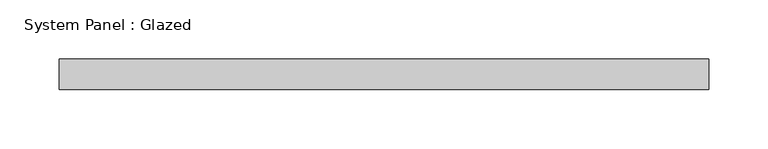
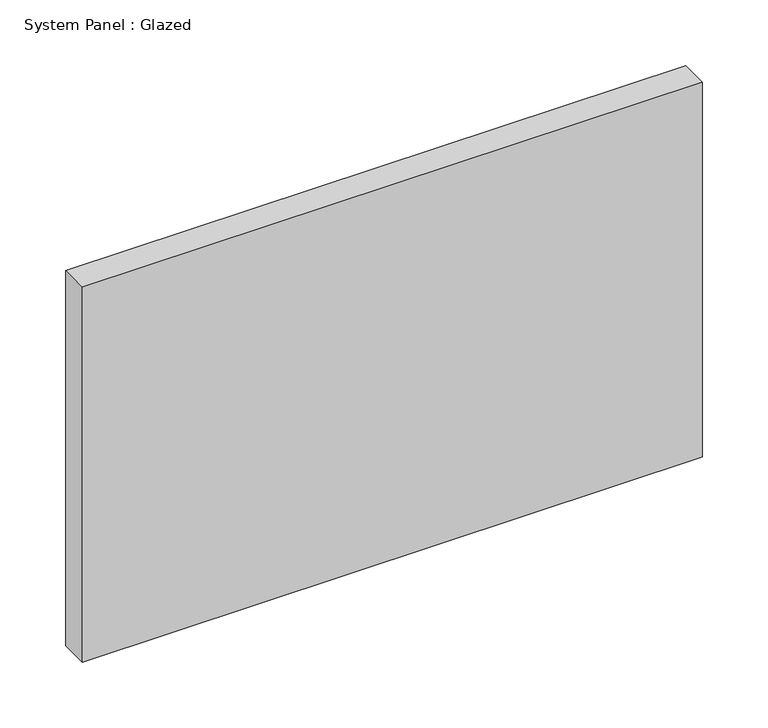
"""IFC4 building model written with IfcOpenShell, lengths in millimetres: plate geometry, System Panel : Glazed."""

from ifc_helpers import new_model, si_unit, origin, origin_with_axes, place, context, project, spatial, polyline, outline, extrude, source, transform, mapped, element, save


def system_panel_glazed_5ecf2d74(model_context):
    return source(origin(), model_context, "Body", "SweptSolid", [
        extrude(outline(polyline([(273.05, 19.05), (-273.05, 19.05), (-273.05, 44.45), (273.05, 44.45), (273.05, 19.05)])), origin_with_axes(), (0.0, 0.0, 1.0), 349.25),
    ])


if __name__ == "__main__":
    model = new_model("IFC4")
    model_context = context("Model", 3, world=origin())
    ifc_project = project(units=[si_unit("LENGTHUNIT", "METRE", prefix="MILLI")], contexts=[model_context])
    site = spatial("IfcSite", under=ifc_project)
    building = spatial("IfcBuilding", under=site)
    placement = place(None, origin())
    system_panel_glazed_shape = system_panel_glazed_5ecf2d74(model_context)
    element("IfcPlate", 1, ObjectType="System Panel : Glazed", at=placement, inside=building, context=model_context, shape_type="MappedRepresentation", body=[
        mapped(system_panel_glazed_shape, transform((0.0, 0.0, 0.0), x_axis=(1.0, 0.0, 0.0), y_axis=(0.0, 1.0, 0.0), z_axis=(0.0, 0.0, 1.0))),
    ])
    save(model, "model.ifc")

# Revit data of these elements
# Type "System Panel : Glazed"
#   Construction Type Id = "GSP4R"
#   Analytic Construction = "1/8 in Pilkington single glazing"
#   Visual Light Transmittance = 0.9
#   Solar Heat Gain Coefficient = 0.86
#   Heat Transfer Coefficient (U) = 1.18115 BTU/(h·ft²·°F)
#   Define Thermal Properties by = 1
# Element 1 (IfcPlate, "System Panel : Glazed")
#   Materials on its faces: "Glass"
# Materials
#   "Glass": class "Glass", colour RGB 0 128 192, transparency 0.75, Description = "Soda Lime Glass", Cost = 0
